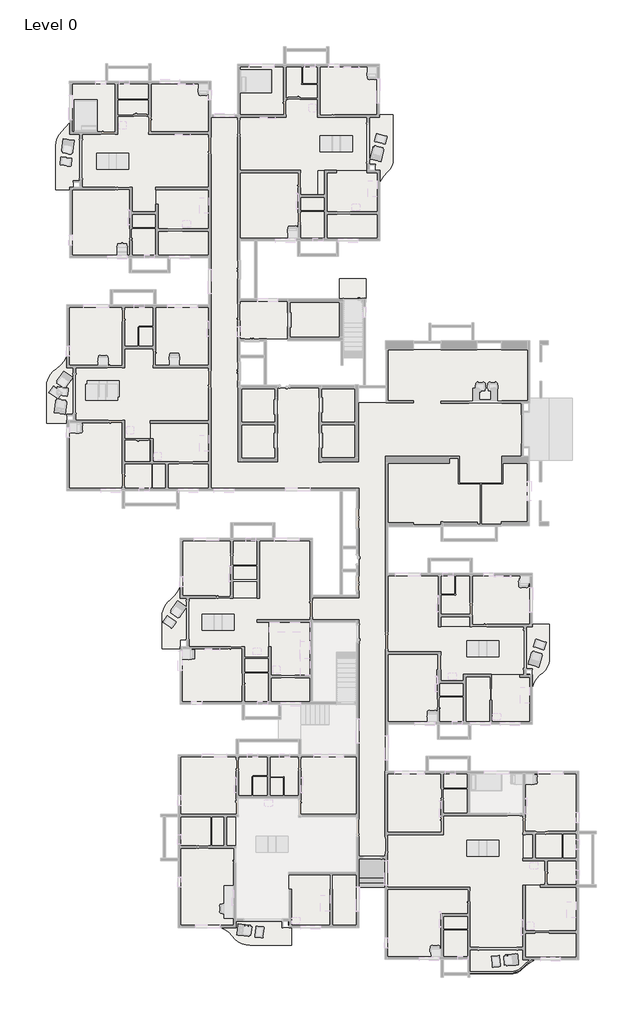
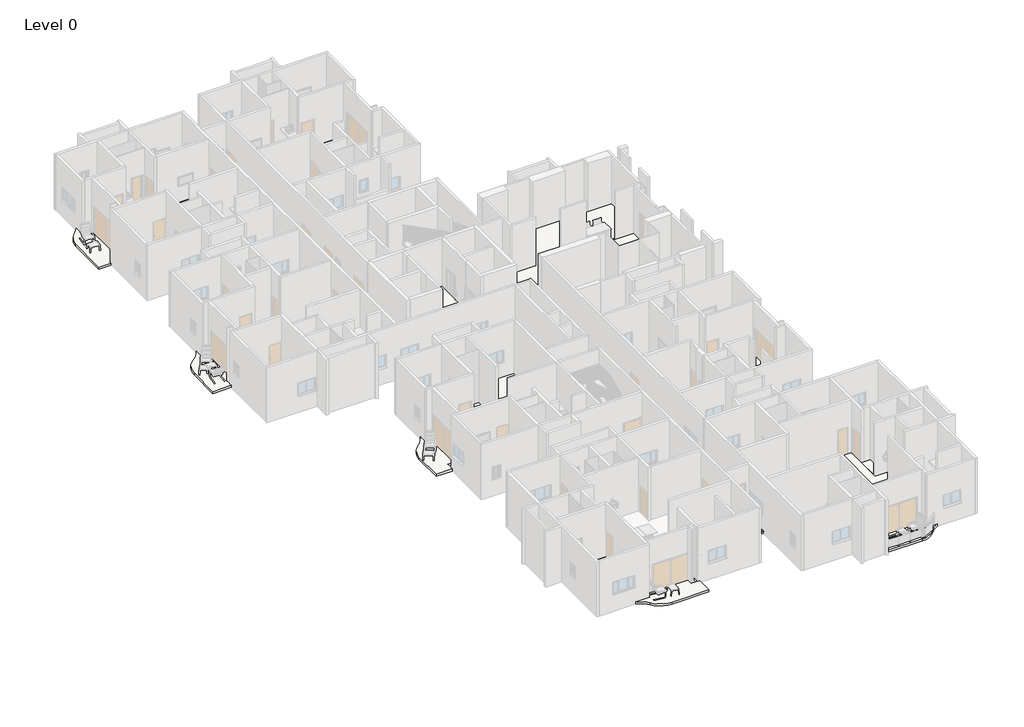
# One storey, part 8 of 14: 11 slabs, 1 stair flight.
"""IFC4 building model written with IfcOpenShell, lengths in millimetres."""

from ifc_helpers import new_model, si_unit, point, frame, frame_2d, origin, origin_with_axes, place, context, project, spatial, polyline, circle_curve, trimmed, segment, composite_curve, outline, extrude, faceted_brep, element, save

model = new_model("IFC4")

# Units and contexts
model_context = context("Model", 3, world=origin())
ifc_project = project(units=[si_unit("LENGTHUNIT", "METRE", prefix="MILLI")], contexts=[model_context])

# Site, building, storey
site = spatial("IfcSite", under=ifc_project)
building = spatial("IfcBuilding", under=site)
storey = spatial("IfcBuildingStorey", under=building, Name="Level 0", Elevation=0.0)

# Slabs
placement = place(None, origin())
element("IfcSlab", 1, at=placement, inside=storey, context=model_context, shape_type="SweptSolid", body=[
    extrude(outline(polyline([(-23242.9901022, 12011.8294818), (-23242.9901022, 15172.0304681), (-21744.3547508, 15172.0304681), (-21744.3547508, 12011.8294818), (-23242.9901022, 12011.8294818)])), origin_with_axes(), (0.0, 0.0, 1.0), 149.9616),
    extrude(outline(polyline([(-11225.1935991, 10026.1220639), (-11225.1935991, 11540.6182059), (-8043.7419991, 11540.6182059), (-8043.7419991, 10026.1220639), (-11225.1935991, 10026.1220639)])), origin_with_axes(), (0.0, 0.0, 1.0), 149.9616),
    extrude(outline(polyline([(-13414.0456172, 27487.7122683), (-13414.0456172, 24693.7122683), (-14938.0456172, 24693.7122683), (-14938.0456172, 27487.7122683), (-13414.0456172, 27487.7122683)])), origin_with_axes(), (0.0, 0.0, 1.0), 149.9616),
    extrude(outline(polyline([(-23595.4772109, 54812.0698597), (-23595.4772109, 56309.0250546), (-20445.8772109, 56309.0250546), (-20445.8772109, 54812.0698597), (-23595.4772109, 54812.0698597)])), origin_with_axes(), (0.0, 0.0, 1.0), 149.9616),
    extrude(outline(polyline([(-34126.2679937, 53766.4998557), (-34126.2679937, 55272.0170169), (-30972.3442282, 55272.0170169), (-30972.3442282, 53766.4998557), (-34126.2679937, 53766.4998557)])), origin_with_axes(), (0.0, 0.0, 1.0), 149.9616),
    extrude(outline(polyline([(-33487.7823022, 39237.6998557), (-33487.7823022, 40756.2978471), (-30972.3442282, 40756.2978471), (-30972.3442282, 39237.6998557), (-33487.7823022, 39237.6998557)])), origin_with_axes(), (0.0, 0.0, 1.0), 149.9616),
    extrude(outline(polyline([(-27067.0691188, 25935.1270746), (-27067.0691188, 27427.6116713), (-24646.9800447, 27427.6116713), (-24646.9800447, 25935.1270746), (-27067.0691188, 25935.1270746)])), origin_with_axes(), (0.0, 0.0, 1.0), 149.9616),
])
element("IfcSlab", 2, at=placement, inside=storey, context=model_context, shape_type="SweptSolid", body=[
    extrude(outline(polyline([(-29269.2063508, 18766.3601529), (-29269.2063508, 16964.8294818), (-29858.3632392, 16964.8294818), (-29858.3632392, 18766.3601529), (-29269.2063508, 18766.3601529)])), origin_with_axes(), (0.0, 0.0, 1.0), 149.9616),
    extrude(outline(polyline([(-11375.5465173, 16175.8530766), (-11375.5465173, 17651.5114683), (-10757.7953327, 17651.5114683), (-10757.7953327, 16175.8530766), (-11375.5465173, 16175.8530766)])), origin_with_axes(), (0.0, 0.0, 1.0), 149.9616),
    extrude(outline(polyline([(-14673.0486976, 31234.1106683), (-14673.0486976, 30624.5106683), (-16476.4486976, 30624.5106683), (-16476.4486976, 31234.1106683), (-14673.0486976, 31234.1106683)])), origin_with_axes(), (0.0, 0.0, 1.0), 149.9616),
    extrude(outline(polyline([(-24164.9149215, 57525.6794361), (-24164.9149215, 59062.4810361), (-23747.8772109, 59062.4810361), (-23747.8772109, 57525.6794361), (-24164.9149215, 57525.6794361)])), origin_with_axes(), (0.0, 0.0, 1.0), 149.9616),
    extrude(outline(polyline([(-35377.7696054, 58008.2998557), (-35377.7696054, 56484.2998557), (-35764.5679937, 56484.2998557), (-35764.5679937, 58008.2998557), (-35377.7696054, 58008.2998557)])), origin_with_axes(), (0.0, 0.0, 1.0), 149.9616),
    extrude(outline(polyline([(-35879.4899915, 47937.0982557), (-35879.4899915, 46762.4498557), (-36204.7442282, 46762.4498557), (-36204.7442282, 47937.0982557), (-35879.4899915, 47937.0982557)])), origin_with_axes(), (0.0, 0.0, 1.0), 149.9616),
    extrude(outline(polyline([(-27953.0447747, 33412.2053139), (-27953.0447747, 32399.4161504), (-29458.4489269, 32399.4161504), (-29458.4489269, 33412.2053139), (-27953.0447747, 33412.2053139)])), origin_with_axes(), (0.0, 0.0, 1.0), 149.9616),
])
element("IfcSlab", 3, at=placement, inside=storey, context=model_context, shape_type="SweptSolid", body=[
    extrude(outline(polyline([(-19777.8949343, 17634.3770397), (-16298.0949343, 17634.3770397), (-16298.0949343, 18845.3114683), (-11375.5465173, 18845.3114683), (-11375.5465173, 16023.4530766), (-9995.7953327, 16023.4530766), (-9995.7953327, 14528.3736639), (-11377.5935991, 14528.3736639), (-11377.5935991, 10628.2590683), (-14663.0433343, 10628.2590683), (-14663.0433343, 14393.9106683), (-19777.8949343, 14393.9106683), (-19777.8949343, 14459.3770397), (-19777.8949343, 17634.3770397)])), origin_with_axes(), (0.0, 0.0, 1.0), 149.9616),
    extrude(outline(polyline([(-11322.6933798, 30624.5106683), (-11322.6933798, 27652.8122683), (-15088.1417798, 27652.8122683), (-15088.1417798, 27259.1122683), (-16485.1417798, 27259.1122683), (-16485.1417798, 29049.8122683), (-19793.4917798, 29049.8122683), (-19793.4917798, 33786.9122683), (-16628.8486976, 33786.9122683), (-16628.8486976, 30624.5106683), (-11322.6933798, 30624.5106683)])), origin_with_axes(), (0.0, 0.0, 1.0), 149.9616),
    extrude(outline(polyline([(-26262.2144411, 65518.2714597), (-26262.2144411, 62540.8795504), (-29018.4788109, 62540.8795504), (-29018.4788109, 65518.2714597), (-26262.2144411, 65518.2714597)])), origin_with_axes(), (0.0, 0.0, 1.0), 149.9616),
    extrude(outline(polyline([(-36809.6998709, 64459.8998557), (-36809.6998709, 61462.6998557), (-39494.1458282, 61462.6998557), (-39494.1458282, 64459.8998557), (-36809.6998709, 64459.8998557)])), origin_with_axes(), (0.0, 0.0, 1.0), 149.9616),
    extrude(outline(polyline([(-26146.3442282, 62364.2982557), (-26146.3442282, 63481.8982557), (-24192.4144411, 63481.8982557), (-24192.4144411, 62338.8982557), (-21119.0144411, 62338.8982557), (-21119.0144411, 59062.4810361), (-24164.9149215, 59062.4810361), (-24164.9149215, 57525.6794361), (-25246.4772109, 57525.6794361), (-25246.4772109, 59062.4810361), (-29018.4788109, 59062.4810361), (-29018.4788109, 62364.2982557), (-26146.3442282, 62364.2982557)])), origin_with_axes(), (0.0, 0.0, 1.0), 149.9616),
    extrude(outline(polyline([(-35751.8679937, 58008.2998557), (-38859.1458282, 58008.2998557), (-38859.1458282, 61310.2998557), (-36657.2998709, 61310.2998557), (-36657.2998709, 62442.0222557), (-34707.2273605, 62442.0222557), (-34707.2273605, 61297.4982557), (-30972.3442282, 61297.4982557), (-30972.3442282, 58008.2998557), (-34278.6679937, 58008.2998557), (-34278.6679937, 56484.2998557), (-35751.8679937, 56484.2998557), (-35751.8679937, 58008.2998557)])), origin_with_axes(), (0.0, 0.0, 1.0), 149.9616),
    extrude(outline(polyline([(-39264.6800447, 46762.4498557), (-36204.7442282, 46762.4498557), (-36204.7442282, 47937.0982557), (-34419.3432055, 47937.0982557), (-34419.3432055, 46768.6982557), (-30972.3442282, 46768.6982557), (-30972.3442282, 43460.4498557), (-34617.3458282, 43460.4498557), (-34617.3458282, 42369.1978471), (-36205.5823022, 42369.1978471), (-36205.5823022, 43479.4998557), (-39264.6800447, 43479.4998557), (-39264.6800447, 46762.4498557)])), origin_with_axes(), (0.0, 0.0, 1.0), 149.9616),
    extrude(outline(polyline([(-32203.4800447, 32382.0541094), (-27800.6447747, 32382.0541094), (-27800.6447747, 35984.9800488), (-24646.9800447, 35984.9800488), (-24646.9800447, 31036.4294818), (-27961.1063508, 31036.4294818), (-27961.1063508, 30884.0294818), (-27219.4691188, 30884.0294818), (-27219.4691188, 28703.6762746), (-28717.3300447, 28703.6762746), (-28717.3300447, 29383.1770746), (-32203.4800447, 29383.1770746), (-32203.4800447, 32382.0541094)])), origin_with_axes(), (0.0, 0.0, 1.0), 149.9616),
])
element("IfcSlab", 4, at=placement, inside=storey, context=model_context, shape_type="SweptSolid", body=[
    extrude(outline(polyline([(-29170.8788109, 62364.2982557), (-29170.8788109, 40900.8738327), (-26683.6805211, 40900.8738327), (-26683.6805211, 45509.2690597), (-24080.1805211, 45509.2690597), (-24080.1805211, 40886.4690597), (-21614.5411875, 40886.4690597), (-21614.5411875, 44569.3674597), (-18194.8375841, 44569.3674597), (-18194.8375841, 44696.4690597), (-19795.0375841, 44696.4690597), (-19795.0375841, 47870.1159129), (-11082.8375841, 47870.1159129), (-11082.8375841, 44695.1159129), (-16467.6375841, 44695.1159129), (-16467.6375841, 44551.7207072), (-11474.7110598, 44551.7207072), (-11474.7110598, 41249.7207072), (-12708.4375841, 41249.7207072), (-12708.4375841, 39561.8923554), (-15346.768917, 39561.8923554), (-15346.768917, 41238.2923554), (-19944.168917, 41238.2923554), (-19944.168917, 16295.4923554), (-21595.168917, 16295.4923554), (-21595.168917, 31027.4923554), (-24494.5800447, 31027.4923554), (-24494.5800447, 32430.4998557), (-21598.9800447, 32430.4998557), (-21598.9800447, 39237.6998557), (-30819.9442282, 39237.6998557), (-30819.9442282, 62364.2982557), (-29170.8788109, 62364.2982557)])), frame((0.0, 0.0, 358.14), z_axis=(0.0, 0.0, 1.0), x_axis=(1.0, 0.0, 0.0)), (0.0, 0.0, 1.0), 149.9616),
])
element("IfcSlab", 5, at=placement, inside=storey, context=model_context, shape_type="SweptSolid", body=[
    extrude(outline(polyline([(-15945.4745014, 40796.435929), (-15945.4745014, 41107.636729), (-15396.146517, 41107.636729), (-15396.146517, 39512.5147554), (-14016.774117, 39512.5147554), (-14016.774117, 37003.2763386), (-14205.4917798, 37003.2763386), (-14205.4917798, 37133.4259386), (-16364.3901798, 37133.4259386), (-16364.3901798, 37152.4759386), (-16491.4917798, 37152.4759386), (-16491.4917798, 36977.8763386), (-18193.2917798, 36977.8763386), (-18193.2917798, 37108.0259386), (-19793.4917798, 37108.0259386), (-19793.4917798, 40796.435929), (-15945.4745014, 40796.435929)])), origin_with_axes(), (0.0, 0.0, 1.0), 149.9616),
    extrude(outline(polyline([(-12627.546517, 39512.5147554), (-12627.546517, 40794.2677015), (-11081.3933798, 40794.2677015), (-11081.3933798, 37158.8259386), (-12706.8917798, 37158.8259386), (-12706.8917798, 37003.2763386), (-13967.396517, 37003.2763386), (-13967.396517, 39512.5147554), (-12627.546517, 39512.5147554)])), origin_with_axes(), (0.0, 0.0, 1.0), 149.9616),
    extrude(outline(polyline([(-26059.2772109, 50906.8706597), (-26039.7911684, 50233.6690597), (-26039.7911684, 49261.8320599), (-26039.7911684, 48570.0706597), (-29018.4788109, 48570.0706597), (-29018.4788109, 50906.8706597), (-26059.2772109, 50906.8706597)])), origin_with_axes(), (0.0, 0.0, 1.0), 149.9616),
])
element("IfcSlab", 6, ObjectType="BALCONY", at=placement, inside=storey, context=model_context, shape_type="SweptSolid", body=[
    extrude(outline(composite_curve([segment(polyline([(-25808.4563508, 10767.2294818), (-28373.8563508, 10767.2294818)]), True, "CONTINUOUS"), segment(trimmed(circle_curve(frame_2d((-28373.8563508, 12172.0434491)), 1404.8139673), [point((-28373.8563508, 10767.2294818))], [point((-29510.8646642, 11346.9892825))], False, "CARTESIAN"), True, "CONTINUOUS"), segment(trimmed(circle_curve(frame_2d((-30660.1207484, 10513.0476923)), 1419.9465211), [point((-29510.8646642, 11346.9892825))], [point((-30209.0063508, 11859.4294818))], True, "CARTESIAN"), True, "CONTINUOUS"), segment(polyline([(-30209.0063508, 11859.4294818), (-29252.4064125, 11859.4294818), (-29252.4064125, 12265.8294818), (-26407.6064125, 12265.8294818), (-26407.6064125, 11859.4294818), (-25808.4563508, 11859.4294818), (-25808.4563508, 10767.2294818)]), True, "CONTINUOUS")], self_intersect=False)), origin_with_axes(), (0.0, 0.0, 1.0), 149.9616),
    extrude(outline(composite_curve([segment(polyline([(-14663.0433343, 8977.2590683), (-14663.0433343, 10475.8590683), (-11377.5935991, 10475.8590683), (-11377.5935991, 9873.7220639), (-10634.5419991, 9873.7220639)]), True, "CONTINUOUS"), segment(trimmed(circle_curve(frame_2d((-9341.4478083, 7424.519782)), 2769.600044), [point((-10634.5419991, 9873.7220639))], [point((-11358.9065962, 9322.029846))], True, "CARTESIAN"), True, "CONTINUOUS"), segment(trimmed(circle_curve(frame_2d((-12156.4858038, 10072.1887005)), 1094.9296322), [point((-11358.9065962, 9322.029846))], [point((-12156.4858038, 8977.2590683))], False, "CARTESIAN"), True, "CONTINUOUS"), segment(polyline([(-12156.4858038, 8977.2590683), (-14663.0433343, 8977.2590683)]), True, "CONTINUOUS")], self_intersect=False)), origin_with_axes(), (0.0, 0.0, 1.0), 149.9616),
    extrude(outline(composite_curve([segment(polyline([(-10782.8417798, 30776.9106683), (-9716.0417798, 30776.9106683), (-9716.0417798, 28667.0901899)]), True, "CONTINUOUS"), segment(trimmed(circle_curve(frame_2d((-10931.4437573, 28667.0901899)), 1215.4019775), [point((-9716.0417798, 28667.0901899))], [point((-10131.2676038, 27752.2568224))], False, "CARTESIAN"), True, "CONTINUOUS"), segment(trimmed(circle_curve(frame_2d((-9303.4618602, 26453.6297898)), 1540.0306877), [point((-10131.2676038, 27752.2568224))], [point((-10789.2933798, 26858.5979543))], True, "CARTESIAN"), True, "CONTINUOUS"), segment(polyline([(-10789.2933798, 26858.5979543), (-10789.2933798, 28025.9106683), (-11170.2933798, 28025.9106683), (-11170.2933798, 30624.5106683), (-10782.8417798, 30624.5106683), (-10782.8417798, 30776.9106683)]), True, "CONTINUOUS")], self_intersect=False)), origin_with_axes(), (0.0, 0.0, 1.0), 149.9616),
    extrude(outline(composite_curve([segment(polyline([(-20312.6288109, 62355.8698597), (-20312.6288109, 62508.2698597), (-19461.7288109, 62508.2698597), (-19461.7288109, 59764.1656665)]), True, "CONTINUOUS"), segment(trimmed(circle_curve(frame_2d((-20564.3341584, 59764.1656665)), 1102.6053475), [point((-19461.7288109, 59764.1656665))], [point((-19804.2864967, 58965.3752657))], False, "CARTESIAN"), True, "CONTINUOUS"), segment(trimmed(circle_curve(frame_2d((-17831.1943737, 56891.7065643)), 2862.3756584), [point((-19804.2864967, 58965.3752657))], [point((-20293.4772109, 58351.2810361))], True, "CARTESIAN"), True, "CONTINUOUS"), segment(polyline([(-20293.4772109, 58351.2810361), (-20293.4772109, 59062.4810361), (-20560.1772109, 59062.4810361), (-20560.1772109, 59460.2698597), (-20953.9788109, 59460.2698597), (-20953.9788109, 62355.8698597), (-20312.6288109, 62355.8698597)]), True, "CONTINUOUS")], self_intersect=False)), origin_with_axes(), (0.0, 0.0, 1.0), 149.9616),
    extrude(outline(composite_curve([segment(polyline([(-39671.9458282, 57855.8998557), (-40510.1458282, 57855.8998557), (-40510.1458282, 60585.4986479)]), True, "CONTINUOUS"), segment(trimmed(circle_curve(frame_2d((-39310.4331095, 60585.4986479)), 1199.7127186), [point((-40510.1458282, 60585.4986479))], [point((-40128.8637104, 61462.6998557))], False, "CARTESIAN"), True, "CONTINUOUS"), segment(trimmed(circle_curve(frame_2d((-42465.254055, 63966.8638371)), 3424.844097), [point((-40128.8637104, 61462.6998557))], [point((-39646.5458282, 62021.4998557))], True, "CARTESIAN"), True, "CONTINUOUS"), segment(polyline([(-39646.5458282, 62021.4998557), (-39646.5458282, 61310.2998557), (-39011.5458282, 61310.2998557), (-39011.5458282, 58396.0966928), (-39413.3013294, 58396.0966928), (-39413.3013294, 58008.2998557), (-39671.9458282, 58008.2998557), (-39671.9458282, 57855.8998557)]), True, "CONTINUOUS")], self_intersect=False)), origin_with_axes(), (0.0, 0.0, 1.0), 149.9616),
    extrude(outline(composite_curve([segment(polyline([(-39810.8816447, 43301.6998557), (-41080.8816447, 43301.6998557), (-41080.8816447, 45539.9441484)]), True, "CONTINUOUS"), segment(trimmed(circle_curve(frame_2d((-39697.8337339, 45539.9441484)), 1383.0479108), [point((-41080.8816447, 45539.9441484))], [point((-40448.2640271, 46701.6996729))], False, "CARTESIAN"), True, "CONTINUOUS"), segment(trimmed(circle_curve(frame_2d((-41570.3708007, 48273.473964)), 1931.2167236), [point((-40448.2640271, 46701.6996729))], [point((-39824.3458282, 47448.2498557))], True, "CARTESIAN"), True, "CONTINUOUS"), segment(polyline([(-39824.3458282, 47448.2498557), (-39824.3458282, 46762.4498557), (-39417.0800447, 46762.4498557), (-39417.0800447, 43847.7998557), (-39810.8816447, 43847.7998557), (-39810.8816447, 43301.6998557)]), True, "CONTINUOUS")], self_intersect=False)), origin_with_axes(), (0.0, 0.0, 1.0), 149.9616),
    extrude(outline(composite_curve([segment(polyline([(-32762.2800447, 29230.7770746), (-33879.8800447, 29230.7770746), (-33879.8800447, 31213.0112133)]), True, "CONTINUOUS"), segment(trimmed(circle_curve(frame_2d((-32483.0499295, 31213.0112133)), 1396.8301152), [point((-33879.8800447, 31213.0112133))], [point((-33350.8197482, 32307.5932854))], False, "CARTESIAN"), True, "CONTINUOUS"), segment(trimmed(circle_curve(frame_2d((-34632.4864875, 33924.2540692)), 2063.0709441), [point((-33350.8197482, 32307.5932854))], [point((-32744.0041796, 33093.6541094))], True, "CARTESIAN"), True, "CONTINUOUS"), segment(polyline([(-32744.0041796, 33093.6541094), (-32744.0041796, 32382.0541094), (-32378.5723524, 32382.0541094), (-32378.5723524, 29791.2541094), (-32762.2800447, 29791.2541094), (-32762.2800447, 29230.7770746)]), True, "CONTINUOUS")], self_intersect=False)), origin_with_axes(), (0.0, 0.0, 1.0), 149.9616),
])
element("IfcSlab", 7, ObjectType="LIFT FLOOR", at=placement, inside=storey, context=model_context, shape_type="SweptSolid", body=[
    extrude(outline(polyline([(-22782.6772109, 50830.6706597), (-22782.6772109, 48652.2320599), (-25861.9911684, 48652.2320599), (-25861.9911684, 50830.6706597), (-22782.6772109, 50830.6706597)])), origin_with_axes(), (0.0, 0.0, 1.0), 149.9616),
    extrude(outline(polyline([(-26838.4514993, 45433.0690597), (-26838.4514993, 43363.3183335), (-28918.8805211, 43363.3183335), (-28918.8805211, 45433.0690597), (-26838.4514993, 45433.0690597)])), origin_with_axes(), (0.0, 0.0, 1.0), 149.9616),
    extrude(outline(polyline([(-26836.0805211, 43210.9183335), (-26836.0805211, 41129.4738327), (-28918.8805211, 41129.4738327), (-28918.8805211, 43210.9183335), (-26836.0805211, 43210.9183335)])), origin_with_axes(), (0.0, 0.0, 1.0), 149.9616),
    extrude(outline(polyline([(-23927.7805211, 41132.9954914), (-23927.7805211, 43210.9183335), (-21843.1411875, 43210.9183335), (-21843.1411875, 41132.9954914), (-23927.7805211, 41132.9954914)])), origin_with_axes(), (0.0, 0.0, 1.0), 149.9616),
    extrude(outline(polyline([(-23927.7805211, 43363.3183335), (-23927.7805211, 45433.0690597), (-21844.9805211, 45433.0690597), (-21844.9805211, 43363.3183335), (-23927.7805211, 43363.3183335)])), origin_with_axes(), (0.0, 0.0, 1.0), 149.9616),
])
element("IfcSlab", 8, ObjectType="OUTDOOR", at=placement, inside=storey, context=model_context, shape_type="SweptSolid", body=[
    extrude(outline(polyline([(-21167.4288686, 52301.6473641), (-21167.4288686, 51059.2706597), (-22808.0772109, 51059.2706597), (-22808.0772109, 52301.6473641), (-21167.4288686, 52301.6473641)])), origin_with_axes(), (0.0, 0.0, 1.0), 149.9616),
])
element("IfcSlab", 9, ObjectType="Toilet floor", at=placement, inside=storey, context=model_context, shape_type="SweptSolid", body=[
    extrude(outline(polyline([(-28740.4522077, 25935.1270746), (-28740.4522077, 28654.2986746), (-27219.4691188, 28654.2986746), (-27219.4691188, 25935.1270746), (-28740.4522077, 25935.1270746)])), origin_with_axes(), (0.0, 0.0, 1.0), 149.9616),
    extrude(outline(polyline([(-27307.2074234, 22512.8601529), (-27307.2074234, 20080.5411882), (-29119.7280604, 20080.5411882), (-29119.7280604, 22512.8601529), (-27307.2074234, 22512.8601529)])), origin_with_axes(), (0.0, 0.0, 1.0), 149.9616),
    extrude(outline(polyline([(-25359.3553928, 22500.1601529), (-25359.3553928, 20080.5411882), (-27154.8074234, 20080.5411882), (-27154.8074234, 22500.1601529), (-25359.3553928, 22500.1601529)])), origin_with_axes(), (0.0, 0.0, 1.0), 149.9616),
    extrude(outline(polyline([(-30010.7632392, 18766.3601529), (-30010.7632392, 16953.9111792), (-32723.5555508, 16953.9111792), (-32723.5555508, 18766.3601529), (-30010.7632392, 18766.3601529)])), origin_with_axes(), (0.0, 0.0, 1.0), 149.9616),
    extrude(outline(polyline([(-27953.0447747, 35984.9800488), (-27953.0447747, 33560.0150638), (-29458.4489269, 33560.0150638), (-29458.4489269, 35984.9800488), (-27953.0447747, 35984.9800488)])), origin_with_axes(), (0.0, 0.0, 1.0), 149.9616),
    extrude(outline(polyline([(-33640.1823022, 40756.2978471), (-33640.1823022, 39237.6998557), (-36205.5823022, 39237.6998557), (-36205.5823022, 40756.2978471), (-33640.1823022, 40756.2978471)])), origin_with_axes(), (0.0, 0.0, 1.0), 149.9616),
    extrude(outline(polyline([(-34419.3432055, 50515.2998557), (-34419.3432055, 48089.4982557), (-36204.7442282, 48089.4982557), (-36204.7442282, 50515.2998557), (-34419.3432055, 50515.2998557)])), origin_with_axes(), (0.0, 0.0, 1.0), 149.9616),
    extrude(outline(polyline([(-34262.7798572, 56331.8998557), (-34262.7798572, 53766.4998557), (-35764.5679937, 53766.4998557), (-35764.5679937, 56331.8998557), (-34262.7798572, 56331.8998557)])), origin_with_axes(), (0.0, 0.0, 1.0), 149.9616),
    extrude(outline(polyline([(-34707.2273605, 64459.8998557), (-34707.2273605, 62516.7998557), (-36657.2998709, 62516.7998557), (-36657.2998709, 64459.8998557), (-34707.2273605, 64459.8998557)])), origin_with_axes(), (0.0, 0.0, 1.0), 149.9616),
    extrude(outline(polyline([(-24205.1144411, 65518.2714597), (-24205.1144411, 63575.1714597), (-26160.9144411, 63575.1714597), (-26160.9144411, 65518.2714597), (-24205.1144411, 65518.2714597)])), origin_with_axes(), (0.0, 0.0, 1.0), 149.9616),
    extrude(outline(polyline([(-23747.8772109, 57373.2794361), (-23747.8772109, 54812.0698597), (-25246.4772109, 54812.0698597), (-25246.4772109, 57373.2794361), (-23747.8772109, 57373.2794361)])), origin_with_axes(), (0.0, 0.0, 1.0), 149.9616),
    extrude(outline(polyline([(-14673.0486976, 33786.9122683), (-14673.0486976, 31386.5106683), (-16476.4486976, 31386.5106683), (-16476.4486976, 33786.9122683), (-14673.0486976, 33786.9122683)])), origin_with_axes(), (0.0, 0.0, 1.0), 149.9616),
    extrude(outline(polyline([(-15062.0602348, 27104.561205), (-15062.0602348, 24693.7122683), (-16598.2323876, 24693.7122683), (-16598.2323876, 27104.561205), (-15062.0602348, 27104.561205)])), origin_with_axes(), (0.0, 0.0, 1.0), 149.9616),
    extrude(outline(polyline([(-14822.8537173, 21442.5122683), (-14822.8537173, 19025.5788751), (-16339.6741157, 19025.5788751), (-16339.6741157, 21442.5122683), (-14822.8537173, 21442.5122683)])), origin_with_axes(), (0.0, 0.0, 1.0), 149.9616),
    extrude(outline(polyline([(-14815.4433343, 12569.4999087), (-14815.4433343, 10005.7106683), (-16324.4276027, 10005.7106683), (-16324.4276027, 12569.4999087), (-14815.4433343, 12569.4999087)])), origin_with_axes(), (0.0, 0.0, 1.0), 149.9616),
    extrude(outline(polyline([(-10605.3953327, 16175.8530766), (-10605.3953327, 17671.826175), (-8039.9933343, 17671.826175), (-8039.9933343, 16175.8530766), (-10605.3953327, 16175.8530766)])), origin_with_axes(), (0.0, 0.0, 1.0), 149.9616),
    extrude(outline(polyline([(-9843.3953327, 14528.3736639), (-9843.3953327, 16023.4530766), (-8039.9933343, 16023.4530766), (-8039.9933343, 14528.3736639), (-9843.3953327, 14528.3736639)])), origin_with_axes(), (0.0, 0.0, 1.0), 149.9616),
    extrude(outline(polyline([(-34592.7839022, 42273.9986471), (-34592.7839022, 40908.6978471), (-36205.5823022, 40908.6978471), (-36205.5823022, 42273.9986471), (-34592.7839022, 42273.9986471)])), origin_with_axes(), (0.0, 0.0, 1.0), 149.9616),
])
element("IfcSlab", 10, ObjectType="bedroom floor", at=placement, inside=storey, context=model_context, shape_type="SweptSolid", body=[
    extrude(outline(polyline([(-29421.6063508, 16801.5111792), (-29421.6063508, 12011.8294818), (-32723.5555508, 12011.8294818), (-32723.5555508, 16801.5111792), (-29421.6063508, 16801.5111792)])), origin_with_axes(), (0.0, 0.0, 1.0), 149.9616),
    extrude(outline(polyline([(-29221.0280604, 22500.1601529), (-29221.0280604, 18908.8981245), (-32723.5555508, 18908.8981245), (-32723.5555508, 22500.1601529), (-29221.0280604, 22500.1601529)])), origin_with_axes(), (0.0, 0.0, 1.0), 149.9616),
    extrude(outline(polyline([(-25206.9553928, 22500.1601529), (-21744.3547508, 22500.1601529), (-21744.3547508, 18872.9762656), (-25206.9553928, 18872.9762656), (-25206.9553928, 22500.1601529)])), origin_with_axes(), (0.0, 0.0, 1.0), 149.9616),
    extrude(outline(polyline([(-16476.8276027, 14241.5106683), (-14739.2433343, 14241.5106683), (-14739.2433343, 12721.8999087), (-16476.8276027, 12721.8999087), (-16476.8276027, 10050.5106683), (-19812.9949343, 10050.5106683), (-19812.9949343, 14241.5106683), (-16476.8276027, 14241.5106683)])), origin_with_axes(), (0.0, 0.0, 1.0), 149.9616),
    extrude(outline(polyline([(-16453.6741156, 21442.5122683), (-16453.6741156, 17829.5106683), (-19812.9949343, 17829.5106683), (-19812.9949343, 21442.5122683), (-16453.6741156, 21442.5122683)])), origin_with_axes(), (0.0, 0.0, 1.0), 149.9616),
    extrude(outline(polyline([(-11223.1465173, 17830.299424), (-11223.1465173, 21442.5122683), (-8039.9933343, 21442.5122683), (-8039.9933343, 17830.299424), (-11223.1465173, 17830.299424)])), origin_with_axes(), (0.0, 0.0, 1.0), 149.9616),
    extrude(outline(polyline([(-16716.0456172, 28897.4122683), (-16716.0456172, 24693.7122683), (-19793.4917798, 24693.7122683), (-19793.4917798, 28897.4122683), (-16716.0456172, 28897.4122683)])), origin_with_axes(), (0.0, 0.0, 1.0), 149.9616),
    extrude(outline(polyline([(-10935.2417798, 33786.9122683), (-10935.2417798, 30776.9106683), (-14520.6486976, 30776.9106683), (-14520.6486976, 33786.9122683), (-10935.2417798, 33786.9122683)])), origin_with_axes(), (0.0, 0.0, 1.0), 149.9616),
    extrude(outline(polyline([(-25398.8772109, 58910.0810361), (-25398.8772109, 54812.0698597), (-29018.4788109, 54812.0698597), (-29018.4788109, 58910.0810361), (-25398.8772109, 58910.0810361)])), origin_with_axes(), (0.0, 0.0, 1.0), 149.9616),
    extrude(outline(polyline([(-24040.0144411, 62508.2698597), (-24040.0144411, 65518.2714597), (-20465.0288109, 65518.2714597), (-20465.0288109, 62508.2698597), (-24040.0144411, 62508.2698597)])), origin_with_axes(), (0.0, 0.0, 1.0), 149.9616),
    extrude(outline(polyline([(-34554.8273605, 61449.8982557), (-34554.8273605, 64459.8998557), (-30972.3442282, 64459.8998557), (-30972.3442282, 61449.8982557), (-34554.8273605, 61449.8982557)])), origin_with_axes(), (0.0, 0.0, 1.0), 149.9616),
    extrude(outline(polyline([(-35904.2679937, 57855.8998557), (-35904.2679937, 53766.4998557), (-39494.1458282, 53766.4998557), (-39494.1458282, 57855.8998557), (-35904.2679937, 57855.8998557)])), origin_with_axes(), (0.0, 0.0, 1.0), 149.9616),
    extrude(outline(polyline([(-36357.1442282, 50515.2998557), (-36357.1442282, 46914.8498557), (-39671.9458282, 46914.8498557), (-39671.9458282, 50515.2998557), (-36357.1442282, 50515.2998557)])), origin_with_axes(), (0.0, 0.0, 1.0), 149.9616),
    extrude(outline(polyline([(-30972.3442282, 50515.2998557), (-30972.3442282, 46921.0982557), (-34266.9432055, 46921.0982557), (-34266.9432055, 50515.2998557), (-30972.3442282, 50515.2998557)])), origin_with_axes(), (0.0, 0.0, 1.0), 149.9616),
    extrude(outline(polyline([(-36357.9823022, 43327.0998557), (-36357.9823022, 39237.6998557), (-39658.4816447, 39237.6998557), (-39658.4816447, 43327.0998557), (-36357.9823022, 43327.0998557)])), origin_with_axes(), (0.0, 0.0, 1.0), 149.9616),
    extrude(outline(polyline([(-29604.6005269, 35984.9800488), (-29604.6005269, 32521.4541094), (-32617.0041796, 32521.4541094), (-32617.0041796, 35984.9800488), (-29604.6005269, 35984.9800488)])), origin_with_axes(), (0.0, 0.0, 1.0), 149.9616),
    extrude(outline(polyline([(-28869.7300447, 29230.7770746), (-28869.7300447, 25935.1270746), (-32609.8800447, 25935.1270746), (-32609.8800447, 29230.7770746), (-28869.7300447, 29230.7770746)])), origin_with_axes(), (0.0, 0.0, 1.0), 149.9616),
])
element("IfcSlab", 11, ObjectType="kitchen floor", at=placement, inside=storey, context=model_context, shape_type="SweptSolid", body=[
    extrude(outline(polyline([(-11225.1935991, 11663.0633156), (-11225.1935991, 14509.3236639), (-8043.7419991, 14509.3236639), (-8043.7419991, 11663.0633156), (-11225.1935991, 11663.0633156)])), origin_with_axes(), (0.0, 0.0, 1.0), 149.9616),
    extrude(outline(polyline([(-25975.6710986, 12011.8294818), (-25975.6710986, 15324.4304681), (-23395.3901022, 15324.4304681), (-23395.3901022, 12011.8294818), (-25975.6710986, 12011.8294818)])), origin_with_axes(), (0.0, 0.0, 1.0), 149.9616),
    extrude(outline(polyline([(-13344.0940172, 24693.7122683), (-13344.0940172, 27640.1122683), (-10928.8917798, 27640.1122683), (-10928.8917798, 24693.7122683), (-13344.0940172, 24693.7122683)])), origin_with_axes(), (0.0, 0.0, 1.0), 149.9616),
    extrude(outline(polyline([(-23747.8772109, 56461.4250546), (-23747.8772109, 59062.4810361), (-20445.8772109, 59062.4810361), (-20445.8772109, 56461.4250546), (-23747.8772109, 56461.4250546)])), origin_with_axes(), (0.0, 0.0, 1.0), 149.9616),
    extrude(outline(polyline([(-34261.7458282, 55424.4170169), (-34261.7458282, 58008.2998557), (-30972.3442282, 58008.2998557), (-30972.3442282, 55424.4170169), (-34261.7458282, 55424.4170169)])), origin_with_axes(), (0.0, 0.0, 1.0), 149.9616),
    extrude(outline(polyline([(-34617.3458282, 40908.6978471), (-34617.3458282, 43460.4498557), (-30972.3442282, 43460.4498557), (-30972.3442282, 40908.6978471), (-34617.3458282, 40908.6978471)])), origin_with_axes(), (0.0, 0.0, 1.0), 149.9616),
    extrude(outline(polyline([(-27219.4691188, 27580.0116713), (-27219.4691188, 30960.2294818), (-24646.9800447, 30960.2294818), (-24646.9800447, 27580.0116713), (-27219.4691188, 27580.0116713)])), origin_with_axes(), (0.0, 0.0, 1.0), 149.9616),
])

# Stair flight
element("IfcStairFlight", 12, ObjectType="1mm_Tread-175mm_Depth", at=placement, inside=storey, context=model_context, shape_type="SolidModel", body=[
    faceted_brep([(-21591.9547508, 14666.9606683, 165.6666667), (-21591.9547508, 14374.8606683, 165.6666667), (-19965.3949343, 14374.8606683, 165.6666667), (-19965.3949343, 14666.9606683, 165.6666667), (-21591.9547508, 14666.9606683, 0.0), (-21591.9547508, 14374.8606683, 0.0), (-19965.3949343, 14374.8606683, 0.0), (-19965.3949343, 14666.9606683, 0.0), (-21591.9547508, 14959.3770397, 332.3333333), (-21591.9547508, 14666.9606683, 332.3333333), (-19965.3949343, 14666.9606683, 332.3333333), (-19965.3949343, 14959.3770397, 332.3333333), (-21591.9547508, 14959.3770397, 130.8772295), (-21591.9547508, 14729.8773898, 0.0), (-19965.3949343, 14729.8773898, 0.0), (-19965.3949343, 14959.3770397, 130.8772295), (-21591.9547508, 14959.3770397, 499.0), (-19965.3949343, 14959.3770397, 499.0), (-19965.3949343, 15298.0273027, 499.0), (-19965.3949343, 16148.843411, 499.0), (-21591.9547508, 16148.843411, 499.0), (-21591.9547508, 15298.0273027, 499.0), (-21591.9547508, 16148.843411, 324.0), (-21591.9547508, 15298.0273027, 324.0), (-19965.3949343, 15298.0273027, 324.0), (-19965.3949343, 16148.843411, 324.0)], [[[0, 1, 2, 3]], [[1, 0, 4, 5]], [[2, 1, 5, 6]], [[3, 2, 6, 7]], [[8, 9, 10, 11]], [[4, 0, 9, 8, 12, 13]], [[0, 3, 10, 9]], [[3, 7, 14, 15, 11, 10]], [[16, 17, 18, 19, 20, 21]], [[8, 16, 21, 20, 22, 23, 12]], [[8, 11, 17, 16]], [[17, 11, 15, 24, 25, 19, 18]], [[20, 19, 25, 22]], [[5, 4, 13, 14, 7, 6]], [[23, 24, 15, 14, 13, 12]], [[24, 23, 22, 25]]]),
    extrude(outline(polyline([(-21591.9547508, 14666.9606683), (-19965.3949343, 14666.9606683), (-19965.3949343, 14374.8606683), (-21591.9547508, 14374.8606683), (-21591.9547508, 14666.9606683)])), frame((0.0, 0.0, 165.6666667), z_axis=(0.0, 0.0, 1.0), x_axis=(1.0, 0.0, 0.0)), (0.0, 0.0, 1.0), 1.0),
    extrude(outline(polyline([(-21591.9547508, 14959.3770397), (-19965.3949343, 14959.3770397), (-19965.3949343, 14666.9606683), (-21591.9547508, 14666.9606683), (-21591.9547508, 14959.3770397)])), frame((0.0, 0.0, 332.3333333), z_axis=(0.0, 0.0, 1.0), x_axis=(1.0, 0.0, 0.0)), (0.0, 0.0, 1.0), 1.0),
    extrude(outline(polyline([(-21591.9547508, 16148.843411), (-19965.3949343, 16148.843411), (-19965.3949343, 14959.3770397), (-21591.9547508, 14959.3770397), (-21591.9547508, 16148.843411)])), frame((0.0, 0.0, 499.0), z_axis=(0.0, 0.0, 1.0), x_axis=(1.0, 0.0, 0.0)), (0.0, 0.0, 1.0), 1.0),
])

save(model, "model.ifc")

# Revit data of these elements
# Type
#   Function = 0
#   Layers, outside or top first: 21.946 mm "UTILITY AREA" (function 5); 128.016 mm "Structure, Timber Joist/Rafter Layer" (function 1)
# Type
#   Function = 0
#   Layers, outside or top first: 21.946 mm "KITCHEN" (function 5); 128.016 mm "Structure, Timber Joist/Rafter Layer" (function 1)
# Type
#   Function = 0
# Type "BALCONY"
#   Function = 0
#   Layers, outside or top first: 21.946 mm "Wood Planks" (function 5); 128.016 mm "Structure, Timber Joist/Rafter Layer" (function 1)
# Type "LIFT FLOOR"
#   Function = 0
#   Layers, outside or top first: 21.946 mm "lift flooring" (function 5); 128.016 mm "Structure, Timber Joist/Rafter Layer" (function 1)
# Type "OUTDOOR"
#   Function = 0
#   Layers, outside or top first: 21.946 mm "OUTDOOR FLOORING" (function 5); 128.016 mm "Structure, Timber Joist/Rafter Layer" (function 1)
# Type "Toilet floor"
#   Function = 0
#   Layers, outside or top first: 21.946 mm "TOILET" (function 5); 128.016 mm "Structure, Timber Joist/Rafter Layer" (function 1)
# Type "bedroom floor"
#   Function = 0
#   Layers, outside or top first: 21.946 mm "KITCHEN" (function 5); 128.016 mm "Structure, Timber Joist/Rafter Layer" (function 1)
# Type "kitchen floor"
#   Function = 0
#   Layers, outside or top first: 21.946 mm "KITCHEN" (function 5); 128.016 mm "Structure, Timber Joist/Rafter Layer" (function 1)
# Element 1 (IfcSlab)
#   built-in parameter 1001955 = 3.14159 (stored number, unit not read)
#   Height Offset From Level = 149.962 mm
#   Phase Created = New Construction
#   Materials on its faces: "Structure, Timber Joist/Rafter Layer", "UTILITY AREA"
# Element 2 (IfcSlab)
#   Height Offset From Level = 149.962 mm
#   Phase Created = New Construction
#   Materials on its faces: "Structure, Timber Joist/Rafter Layer", "KITCHEN"
# Element 3 (IfcSlab)
#   built-in parameter 1001955 = 1.5708 (stored number, unit not read)
#   Height Offset From Level = 149.962 mm
#   Phase Created = New Construction
#   Materials on its faces: "Structure, Timber Joist/Rafter Layer", "KITCHEN"
# Element 4 (IfcSlab)
#   Height Offset From Level = 508.102 mm
#   Phase Created = New Construction
#   Materials on its faces: "Structure, Timber Joist/Rafter Layer"
# Element 5 (IfcSlab)
#   Height Offset From Level = 149.962 mm
#   Phase Created = New Construction
#   Materials on its faces: "Structure, Timber Joist/Rafter Layer"
# Element 6 (IfcSlab, "BALCONY")
#   built-in parameter 1001955 = -1.5708 (stored number, unit not read)
#   Height Offset From Level = 149.962 mm
#   Phase Created = New Construction
#   Materials on its faces: "Structure, Timber Joist/Rafter Layer", "Wood Planks"
# Element 7 (IfcSlab, "LIFT FLOOR")
#   Height Offset From Level = 149.962 mm
#   Phase Created = New Construction
#   Materials on its faces: "Structure, Timber Joist/Rafter Layer", "lift flooring"
# Element 8 (IfcSlab, "OUTDOOR")
#   Height Offset From Level = 149.962 mm
#   Phase Created = New Construction
#   Materials on its faces: "Structure, Timber Joist/Rafter Layer", "OUTDOOR FLOORING"
# Element 9 (IfcSlab, "Toilet floor")
#   built-in parameter 1001955 = 3.14159 (stored number, unit not read)
#   Height Offset From Level = 149.962 mm
#   Phase Created = New Construction
#   Materials on its faces: "Structure, Timber Joist/Rafter Layer", "TOILET"
# Element 10 (IfcSlab, "bedroom floor")
#   Height Offset From Level = 149.962 mm
#   Phase Created = New Construction
#   Materials on its faces: "Structure, Timber Joist/Rafter Layer", "KITCHEN"
# Element 11 (IfcSlab, "kitchen floor")
#   built-in parameter 1001955 = 3.14159 (stored number, unit not read)
#   Height Offset From Level = 149.962 mm
#   Phase Created = New Construction
#   Materials on its faces: "Structure, Timber Joist/Rafter Layer", "KITCHEN"
# Element 12 (IfcStairFlight, "1mm_Tread-175mm_Depth")
#   Phase Created = New Construction
#   Materials on its faces: "Concrete, Cast-in-Place gray"
# Materials
#   "UTILITY AREA": class "Generic", colour RGB 120 120 120, transparency 0, Cost = 0
#   "Structure, Timber Joist/Rafter Layer": class "Wood", colour RGB 127 127 127, transparency 0, Description = "Timber framing, thermal airspace", Cost = 0
#   "KITCHEN": class "Generic", colour RGB 120 120 120, transparency 0, Cost = 0
#   "Wood Planks": class "Wood", colour RGB 193 160 115, transparency 0, Description = "Physical material.", Cost = 0
#   "lift flooring": class "Generic", colour RGB 120 120 120, transparency 0, Cost = 0
#   "OUTDOOR FLOORING": class "Generic", colour RGB 120 120 120, transparency 0, Cost = 0
#   "TOILET": class "Generic", colour RGB 120 120 120, transparency 0, Cost = 0
#   "Concrete, Cast-in-Place gray": class "Concrete", colour RGB 192 192 192, transparency 0, Description = "Cast-in-place concrete", Cost = 0
